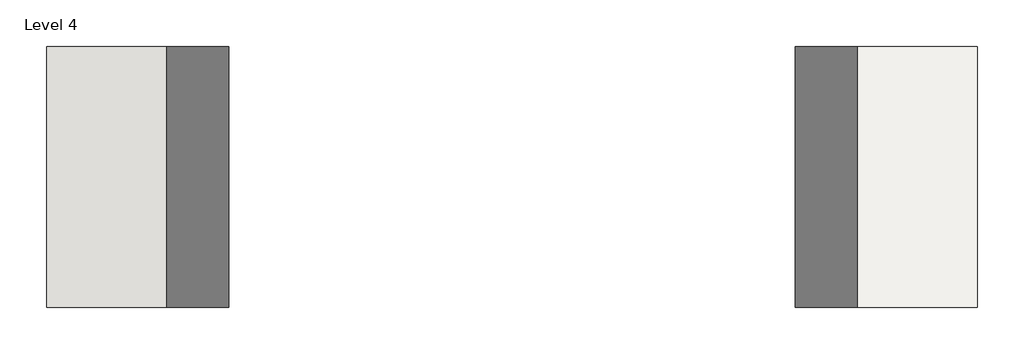
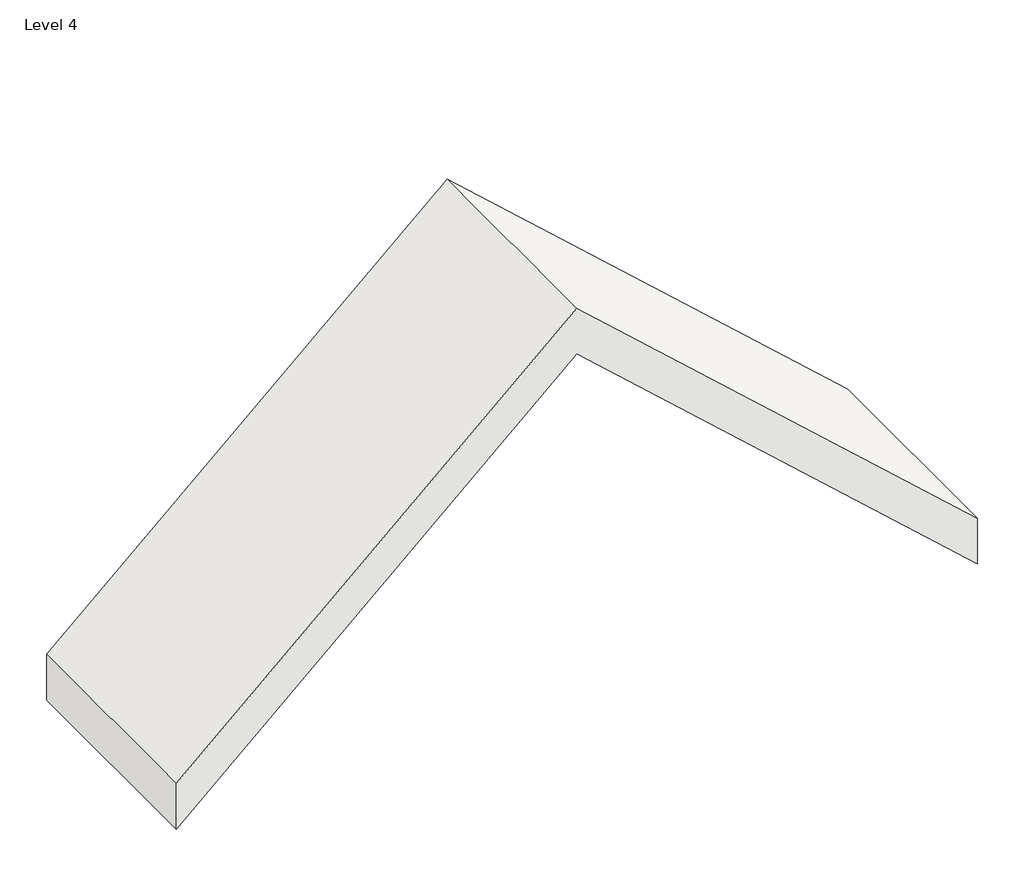
# One storey: 1 roof.
"""IFC4 building model written with IfcOpenShell, lengths in millimetres."""

from ifc_helpers import new_model, si_unit, frame, origin, place, context, project, spatial, polyline, outline, extrude, element, save

model = new_model("IFC4")

# Units and contexts
model_context = context("Model", 3, world=origin())
ifc_project = project(units=[si_unit("LENGTHUNIT", "METRE", prefix="MILLI")], contexts=[model_context])

# Site, building, storey
site = spatial("IfcSite", under=ifc_project)
building = spatial("IfcBuilding", under=site)
storey = spatial("IfcBuildingStorey", under=building, Name="Level 4", Elevation=9144.0)

# Roof
placement = place(None, origin())
element("IfcRoof", 1, ObjectType="Generic - 12\"", at=placement, inside=storey, context=model_context, shape_type="SweptSolid", body=[
    extrude(outline(polyline([(9554.9052989, -2913.676852), (12623.8526318, -6308.1216094), (9554.9052989, -9702.5663667), (9144.0, -9702.5663667), (12212.9473328, -6308.1216094), (9144.0, -2913.676852), (9554.9052989, -2913.676852)])), frame((0.0, -12258.2777232, 0.0), z_axis=(0.0, 1.0, 0.0), x_axis=(0.0, 0.0, 1.0)), (0.0, 0.0, 1.0), 1905.0),
])

save(model, "model.ifc")

# Revit data of these elements
# Type "Generic - 12\""
#   Assembly Code = "B1020"
#   Layers, outside or top first: 1' - 0" no material (function 1)
# Element 1 (IfcRoof, "Generic - 12\"")
#   built-in parameter 1001705 = 41.4168 (stored number, unit not read)
#   built-in parameter 1001710 = 33615
#   Phase Created = New Construction
#   Materials on its faces: "Default Roof"
# Materials
#   "Default Roof": colour RGB 88 101 114, transparency 0, Cost = 0
